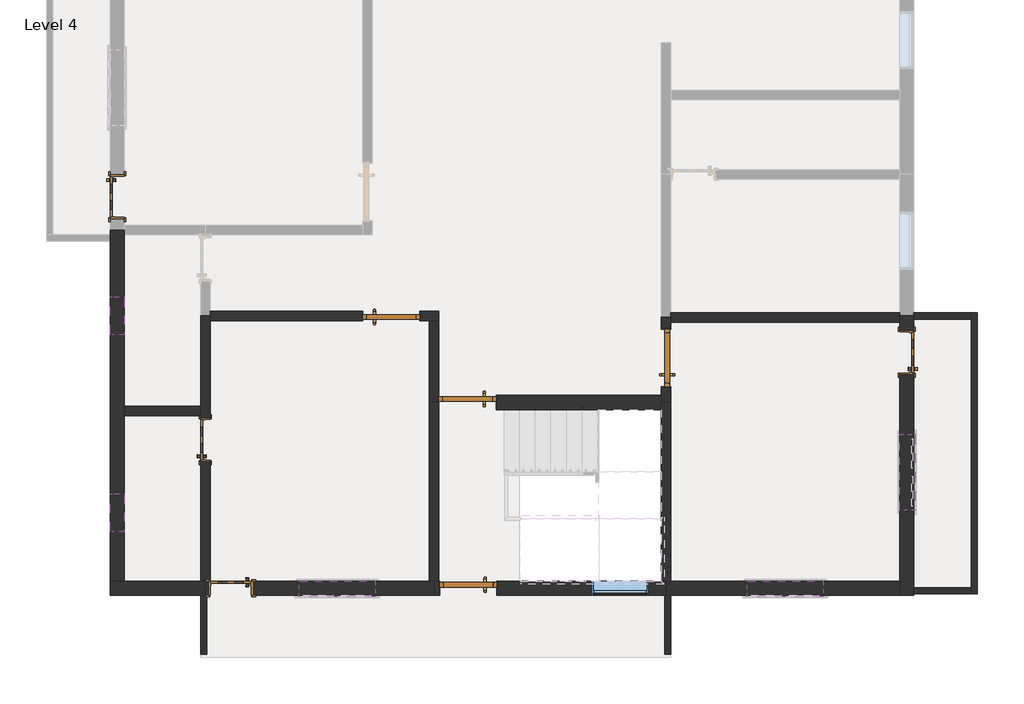
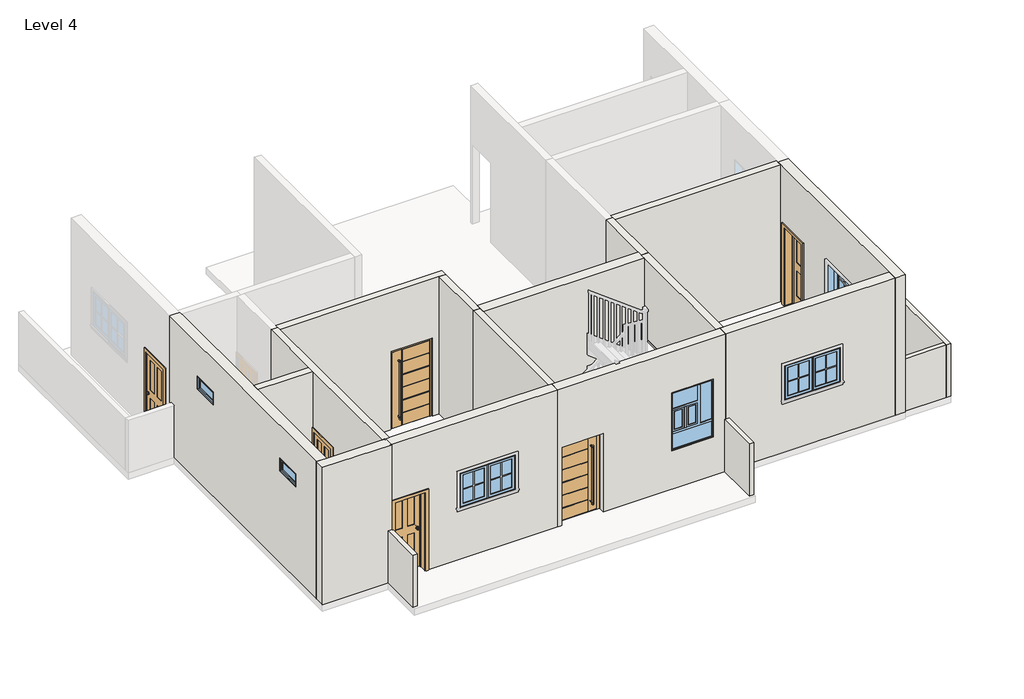
# One storey, part 1 of 3: 20 walls, 8 doors, 6 windows.
"""IFC4 building model written with IfcOpenShell, lengths in millimetres."""

from ifc_helpers import new_model, si_unit, frame, origin, place, context, project, spatial, polyline, outline, extrude, faceted_brep, transform, mapped, element, save
from components import door_3_44036f4b, door_3_3562bf2b, door_a03dd1d4, door_a34dad57, m_fixed_2_dd9f9b20, m_window_awning_double_horizontal_4_8afcb0b2, m_window_casement_double_sash_variable_3_661e274a

model = new_model("IFC4")

# Units and contexts
model_context = context("Model", 3, world=origin())
ifc_project = project(units=[si_unit("LENGTHUNIT", "METRE", prefix="MILLI")], contexts=[model_context])

# Site, building, storey
site = spatial("IfcSite", under=ifc_project)
building = spatial("IfcBuilding", under=site)
storey = spatial("IfcBuildingStorey", under=building, Name="Level 4", Elevation=9601.2)

# Doors
placement = place(None, origin())
door_3_shape = door_3_44036f4b(model_context)
element("IfcDoor", 1, ObjectType="3'", at=placement, inside=storey, context=model_context, shape_type="MappedRepresentation", body=[
    mapped(door_3_shape, transform((-13795.5794909, -9.3618509, 9601.2), x_axis=(1.0, 0.0, 0.0), y_axis=(0.0, 1.0, 0.0), z_axis=(0.0, 0.0, 1.0))),
])
element("IfcDoor", 2, ObjectType="3'", at=placement, inside=storey, context=model_context, shape_type="MappedRepresentation", body=[
    mapped(door_3_shape, transform((-9401.3794909, -682.4618509, 9601.2), x_axis=(0.0, 1.0, 0.0), y_axis=(-1.0, 0.0, 0.0), z_axis=(0.0, 0.0, 1.0))),
])
door_3_2_shape = door_3_3562bf2b(model_context)
element("IfcDoor", 3, ObjectType="3'", at=placement, inside=storey, context=model_context, shape_type="MappedRepresentation", body=[
    mapped(door_3_2_shape, transform((-12576.3794909, -1393.6618509, 9601.2), x_axis=(-1.0, 0.0, 0.0), y_axis=(0.0, -1.0, 0.0), z_axis=(0.0, 0.0, 1.0))),
])
element("IfcDoor", 4, ObjectType="3'", at=placement, inside=storey, context=model_context, shape_type="MappedRepresentation", body=[
    mapped(door_3_2_shape, transform((-12563.6794909, -4365.4618509, 9601.2), x_axis=(-1.0, 0.0, 0.0), y_axis=(0.0, -1.0, 0.0), z_axis=(0.0, 0.0, 1.0))),
])
door_shape = door_a03dd1d4(model_context)
element("IfcDoor", 5, ObjectType="M_Door-Interior-Single-4_Panel-Wood : 2'2\"", at=placement, inside=storey, context=model_context, shape_type="MappedRepresentation", body=[
    mapped(door_shape, transform((-16770.5544909, -1990.1618509, 9601.2), x_axis=(0.0, 1.0, 0.0), y_axis=(-1.0, 0.0, 0.0), z_axis=(0.0, 0.0, 1.0))),
])
door_2_shape = door_a34dad57(model_context)
element("IfcDoor", 6, ObjectType="M_Door-Interior-Single-4_Panel-Wood : 2'2\"", at=placement, inside=storey, context=model_context, shape_type="MappedRepresentation", body=[
    mapped(door_2_shape, transform((-18180.2544909, 1895.2381491, 9601.2), x_axis=(0.0, -1.0, 0.0), y_axis=(1.0, 0.0, 0.0), z_axis=(0.0, 0.0, 1.0))),
])
element("IfcDoor", 7, ObjectType="M_Door-Interior-Single-4_Panel-Wood : 2'2\"", at=placement, inside=storey, context=model_context, shape_type="MappedRepresentation", body=[
    mapped(door_2_shape, transform((-5550.1044909, -593.1618509, 9601.2), x_axis=(0.0, 1.0, 0.0), y_axis=(-1.0, 0.0, 0.0), z_axis=(0.0, 0.0, 1.0))),
])
element("IfcDoor", 8, ObjectType="M_Door-Interior-Single-4_Panel-Wood : 2'2\"", at=placement, inside=storey, context=model_context, shape_type="MappedRepresentation", body=[
    mapped(door_2_shape, transform((-16361.3794909, -4362.2868509, 9601.2), x_axis=(-1.0, 0.0, 0.0), y_axis=(0.0, -1.0, 0.0), z_axis=(0.0, 0.0, 1.0))),
])

# Walls
element("IfcWall", 9, ObjectType="Generic - 4\"", at=placement, inside=storey, context=model_context, shape_type="Brep", body=[
    faceted_brep([(-9325.1794909, -5419.5618509, 9601.2), (-9325.1794909, -4479.7618509, 9601.2), (-9325.1794909, -4479.7618509, 10820.4), (-9325.1794909, -5419.5618509, 10820.4), (-9426.7794909, -5419.5618509, 9601.2), (-9426.7794909, -5419.5618509, 10820.4), (-9426.7794909, -4479.7618509, 10820.4), (-9426.7794909, -4479.7618509, 9601.2), (-9401.3794909, -4479.7618509, 9601.2)], [[[0, 1, 2, 3]], [[4, 5, 6, 7]], [[1, 0, 4, 7, 8]], [[3, 2, 6, 5]], [[0, 3, 5, 4]], [[2, 1, 8, 7, 6]]]),
])
element("IfcWall", 10, ObjectType="Generic - 4\"", at=placement, inside=storey, context=model_context, shape_type="Brep", body=[
    faceted_brep([(-4422.9794909, -4454.3618509, 9601.2), (-4422.9794909, 41.4381491, 9601.2), (-4422.9794909, 41.4381491, 10820.4), (-4422.9794909, -4454.3618509, 10820.4), (-4524.5794909, -4454.3618509, 9601.2), (-4524.5794909, -4454.3618509, 10820.4), (-4524.5794909, -4352.7618509, 10820.4), (-4524.5794909, -60.1618509, 10820.4), (-4524.5794909, 41.4381491, 10820.4), (-4524.5794909, 41.4381491, 9601.2), (-4524.5794909, -60.1618509, 9601.2), (-4524.5794909, -4352.7618509, 9601.2)], [[[0, 1, 2, 3]], [[4, 5, 6, 7, 8, 9, 10, 11]], [[1, 0, 4, 11, 10, 9]], [[3, 2, 8, 7, 6, 5]], [[0, 3, 5, 4]], [[2, 1, 9, 8]]]),
])
element("IfcWall", 11, ObjectType="Generic - 4\"", at=placement, inside=storey, context=model_context, shape_type="SweptSolid", body=[
    extrude(outline(polyline([(-4524.5794909, -4454.3618509), (-5438.9794909, -4454.3618509), (-5438.9794909, -4352.7618509), (-4524.5794909, -4352.7618509), (-4524.5794909, -4454.3618509)])), frame((0.0, 0.0, 9601.2), z_axis=(0.0, 0.0, 1.0), x_axis=(1.0, 0.0, 0.0)), (0.0, 0.0, 1.0), 1219.2),
])
element("IfcWall", 12, ObjectType="Generic - 4\"", at=placement, inside=storey, context=model_context, shape_type="Brep", body=[
    faceted_brep([(-16843.5794909, -4479.7618509, 9601.2), (-16843.5794909, -5419.5618509, 9601.2), (-16843.5794909, -5419.5618509, 10820.4), (-16843.5794909, -4479.7618509, 10820.4), (-16741.9794909, -4479.7618509, 9601.2), (-16741.9794909, -4479.7618509, 10820.4), (-16741.9794909, -5419.5618509, 10820.4), (-16741.9794909, -5419.5618509, 9601.2), (-16792.7794909, -4479.7618509, 9601.2), (-16767.3794909, -4479.7618509, 9601.2)], [[[0, 1, 2, 3]], [[4, 5, 6, 7]], [[1, 0, 8, 9, 4, 7]], [[2, 1, 7, 6]], [[3, 2, 6, 5]], [[0, 3, 5, 4, 9, 8]]]),
])
element("IfcWall", 13, ObjectType="Generic - 4\"", at=placement, inside=storey, context=model_context, shape_type="Brep", body=[
    faceted_brep([(-4524.5794909, 41.4381491, 9601.2), (-5438.9794909, 41.4381491, 9601.2), (-5438.9794909, 41.4381491, 10820.4), (-4524.5794909, 41.4381491, 10820.4), (-4524.5794909, -60.1618509, 9601.2), (-4524.5794909, -60.1618509, 10820.4), (-5438.9794909, -60.1618509, 10820.4), (-5438.9794909, -60.1618509, 9601.2), (-5438.9794909, -34.7618509, 9601.2), (-5438.9794909, -9.3618509, 9601.2)], [[[0, 1, 2, 3]], [[4, 5, 6, 7]], [[1, 0, 4, 7, 8, 9]], [[3, 2, 6, 5]], [[0, 3, 5, 4]], [[2, 1, 9, 8, 7, 6]]]),
])
element("IfcWall", 14, ObjectType="Generic - 6\"", at=placement, inside=storey, context=model_context, shape_type="Brep", body=[
    faceted_brep([(-16691.1794909, -9.3618509, 9601.2), (-16691.1794909, -9.3618509, 12801.6), (-16691.1794909, -85.5618509, 12801.6), (-16691.1794909, -4251.1618509, 12801.6), (-16691.1794909, -4251.1618509, 9601.2), (-16691.1794909, -2345.3618509, 9601.2), (-16691.1794909, -2345.3618509, 11455.0), (-16691.1794909, -1634.9618509, 11455.0), (-16691.1794909, -1634.9618509, 9601.2), (-16691.1794909, -85.5618509, 9601.2), (-16843.5794909, -9.3618509, 12801.6), (-16843.5794909, -9.3618509, 9601.2), (-16843.5794909, -1457.1618509, 9601.2), (-16843.5794909, -1609.5618509, 9601.2), (-16843.5794909, -1634.9618509, 9601.2), (-16843.5794909, -1634.9618509, 11455.0), (-16843.5794909, -2345.3618509, 11455.0), (-16843.5794909, -2345.3618509, 9601.2), (-16843.5794909, -4251.1618509, 9601.2), (-16843.5794909, -4251.1618509, 12801.6), (-16843.5794909, -1609.5618509, 12801.6), (-16843.5794909, -1457.1618509, 12801.6), (-16716.5794909, -4251.1618509, 9601.2), (-16767.3794909, -4251.1618509, 9601.2), (-16792.7794909, -4251.1618509, 9601.2), (-16792.7794909, -4251.1618509, 12801.6), (-16767.3794909, -4251.1618509, 12801.6)], [[[0, 1, 2, 3, 4, 5, 6, 7, 8, 9]], [[10, 11, 12, 13, 14, 15, 16, 17, 18, 19, 20, 21]], [[4, 22, 23, 24, 18, 17, 5]], [[11, 0, 9, 8, 14, 13, 12]], [[1, 0, 11, 10]], [[3, 2, 1, 10, 21, 20, 19, 25, 26]], [[7, 15, 14, 8]], [[15, 7, 6, 16]], [[16, 6, 5, 17]], [[3, 26, 25, 19, 18, 24, 23, 22, 4]]]),
])
element("IfcWall", 15, ObjectType="Generic - 6\"", at=placement, inside=storey, context=model_context, shape_type="SweptSolid", body=[
    extrude(outline(polyline([(-16843.5794909, -1609.5618509), (-18062.7794909, -1609.5618509), (-18062.7794909, -1457.1618509), (-16843.5794909, -1457.1618509), (-16843.5794909, -1609.5618509)])), frame((0.0, 0.0, 9601.2), z_axis=(0.0, 0.0, 1.0), x_axis=(1.0, 0.0, 0.0)), (0.0, 0.0, 1.0), 3200.4),
])
element("IfcWall", 16, ObjectType="Generic - 6\"", at=placement, inside=storey, context=model_context, shape_type="Brep", body=[
    faceted_brep([(-13033.5794909, -85.5618509, 12801.6), (-13185.9794909, -85.5618509, 12801.6), (-16691.1794909, -85.5618509, 12801.6), (-16691.1794909, -85.5618509, 9601.2), (-14252.7794909, -85.5618509, 9601.2), (-14252.7794909, -85.5618509, 11430.0), (-13338.3794909, -85.5618509, 11430.0), (-13338.3794909, -85.5618509, 9601.2), (-13185.9794909, -85.5618509, 9601.2), (-13033.5794909, -85.5618509, 9601.2), (-16691.1794909, 66.8381491, 12801.6), (-13033.5794909, 66.8381491, 12801.6), (-13033.5794909, 66.8381491, 9601.2), (-13338.3794909, 66.8381491, 9601.2), (-13338.3794909, 66.8381491, 11430.0), (-14252.7794909, 66.8381491, 11430.0), (-14252.7794909, 66.8381491, 9601.2), (-16691.1794909, 66.8381491, 9601.2), (-13338.3794909, -65.5618509, 9601.2), (-13323.3794909, -65.5618509, 9601.2), (-13323.3794909, 11.4381491, 9601.2), (-13338.3794909, 11.4381491, 9601.2), (-16691.1794909, -9.3618509, 9601.2), (-14252.7794909, 11.4381491, 9601.2), (-14267.7794909, 11.4381491, 9601.2), (-14267.7794909, -65.5618509, 9601.2), (-14252.7794909, -65.5618509, 9601.2), (-16691.1794909, -9.3618509, 12801.6), (-14252.7794909, -65.5618509, 11430.0), (-13338.3794909, -65.5618509, 11430.0), (-13338.3794909, 11.4381491, 11430.0), (-14252.7794909, 11.4381491, 11430.0), (-14267.7794909, -65.5618509, 11445.0), (-14267.7794909, 11.4381491, 11445.0), (-13323.3794909, 11.4381491, 11445.0), (-13323.3794909, -65.5618509, 11445.0)], [[[0, 1, 2, 3, 4, 5, 6, 7, 8, 9]], [[10, 11, 12, 13, 14, 15, 16, 17]], [[12, 9, 8, 7, 18, 19, 20, 21, 13]], [[3, 22, 17, 16, 23, 24, 25, 26, 4]], [[2, 1, 0, 11, 10, 27]], [[3, 2, 27, 10, 17, 22]], [[0, 9, 12, 11]], [[5, 28, 29, 6]], [[14, 30, 31, 15]], [[6, 29, 18, 7]], [[30, 14, 13, 21]], [[28, 5, 4, 26]], [[15, 31, 23, 16]], [[32, 33, 34, 35]], [[35, 34, 20, 19]], [[31, 30, 21, 20, 34, 33, 24, 23]], [[33, 32, 25, 24]], [[29, 28, 26, 25, 32, 35, 19, 18]]]),
])
element("IfcWall", 17, ObjectType="Generic - 6\"", at=placement, inside=storey, context=model_context, shape_type="Brep", body=[
    faceted_brep([(-13185.9794909, -85.5618509, 9601.2), (-13185.9794909, -1393.6618509, 9601.2), (-13185.9794909, -1393.6618509, 12801.6), (-13185.9794909, -85.5618509, 12801.6), (-13033.5794909, -85.5618509, 12801.6), (-13033.5794909, -1279.3618509, 12801.6), (-13033.5794909, -1393.6618509, 12801.6), (-13033.5794909, -1393.6618509, 11430.0), (-13033.5794909, -1393.6618509, 9601.2), (-13033.5794909, -1376.3618508, 9601.2), (-13033.5794909, -1376.3618508, 11430.0), (-13033.5794909, -1376.3618508, 11445.0), (-13033.5794909, -1299.3618508, 11445.0), (-13033.5794909, -1299.3618508, 11430.0), (-13033.5794909, -1299.3618508, 9601.2), (-13033.5794909, -1279.3618508, 9601.2), (-13033.5794909, -85.5618509, 9601.2), (-13048.5794909, -1299.3618508, 9601.2), (-13048.5794909, -1376.3618508, 9601.2), (-13048.5794909, -1376.3618508, 11445.0), (-13048.5794909, -1299.3618508, 11445.0)], [[[0, 1, 2, 3]], [[4, 5, 6, 7, 8, 9, 10, 11, 12, 13, 14, 15, 16]], [[1, 0, 16, 15, 14, 17, 18, 9, 8]], [[2, 1, 8, 7, 6]], [[3, 2, 6, 5, 4]], [[0, 3, 4, 16]], [[19, 20, 12, 11]], [[20, 19, 18, 17]], [[18, 19, 11, 10, 9]], [[20, 17, 14, 13, 12]]]),
])
element("IfcWall", 18, ObjectType="Generic - 6\"", at=placement, inside=storey, context=model_context, shape_type="Brep", body=[
    faceted_brep([(-9325.1794909, -4251.1618509, 12801.6), (-9325.1794909, -4251.1618509, 9601.2), (-9325.1794909, -1393.6618509, 9601.2), (-9325.1794909, -1393.6618509, 12801.6), (-9477.5794909, -4251.1618509, 9601.2), (-9477.5794909, -4251.1618509, 12801.6), (-9477.5794909, -1507.9618509, 12801.6), (-9477.5794909, -1393.6618509, 12801.6), (-9477.5794909, -1393.6618509, 9601.2), (-9477.5794909, -1507.9618509, 9601.2), (-9401.3794909, -4251.1618509, 9601.2), (-9401.3794909, -4251.1618509, 12801.6)], [[[0, 1, 2, 3]], [[4, 5, 6, 7, 8, 9]], [[2, 1, 10, 4, 9, 8]], [[3, 2, 8, 7]], [[0, 3, 7, 6, 5, 11]], [[0, 11, 5, 4, 10, 1]]]),
])
element("IfcWall", 19, ObjectType="Generic - 6\"", at=placement, inside=storey, context=model_context, shape_type="Brep", body=[
    faceted_brep([(-5667.5794909, 41.4381491, 12801.6), (-5667.5794909, 41.4381491, 9601.2), (-9325.1794909, 41.4381491, 9601.2), (-9325.1794909, 41.4381491, 12801.6), (-5667.5794909, -110.9618509, 9601.2), (-5667.5794909, -110.9618509, 12801.6), (-9325.1794909, -110.9618509, 12801.6), (-9325.1794909, -110.9618509, 9601.2), (-5667.5794909, -9.3618509, 9601.2), (-5667.5794909, -34.7618509, 9601.2), (-9325.1794909, -34.7618509, 9601.2), (-9325.1794909, -34.7618509, 12801.6), (-5667.5794909, -34.7618509, 12801.6), (-5667.5794909, -9.3618509, 12801.6)], [[[0, 1, 2, 3]], [[4, 5, 6, 7]], [[2, 1, 8, 9, 4, 7, 10]], [[0, 3, 11, 6, 5, 12, 13]], [[3, 2, 10, 7, 6, 11]], [[0, 13, 12, 5, 4, 9, 8, 1]]]),
])
element("IfcWall", 20, ObjectType="Generic - 6\"", at=placement, inside=storey, context=model_context, shape_type="Brep", body=[
    faceted_brep([(-9325.1794909, -34.7618509, 9601.2), (-9325.1794909, -34.7618509, 12801.6), (-9325.1794909, -110.9618509, 12801.6), (-9325.1794909, -1393.6618509, 12801.6), (-9325.1794909, -1393.6618509, 9601.2), (-9325.1794909, -1139.6618509, 9601.2), (-9325.1794909, -1139.6618509, 11430.0), (-9325.1794909, -225.2618509, 11430.0), (-9325.1794909, -225.2618509, 9601.2), (-9325.1794909, -110.9618509, 9601.2), (-9477.5794909, -34.7618509, 12801.6), (-9477.5794909, -34.7618509, 9601.2), (-9477.5794909, -225.2618509, 9601.2), (-9477.5794909, -225.2618509, 11430.0), (-9477.5794909, -1139.6618509, 11430.0), (-9477.5794909, -1139.6618509, 9601.2), (-9477.5794909, -1279.3618509, 9601.2), (-9477.5794909, -1393.6618509, 9601.2), (-9477.5794909, -1393.6618509, 12801.6), (-9477.5794909, -1279.3618509, 12801.6), (-9345.1794909, -225.2618509, 9601.2), (-9345.1794909, -210.2618509, 9601.2), (-9422.1794909, -210.2618509, 9601.2), (-9422.1794909, -225.2618509, 9601.2), (-9422.1794909, -1139.6618509, 9601.2), (-9422.1794909, -1154.6618509, 9601.2), (-9345.1794909, -1154.6618509, 9601.2), (-9345.1794909, -1139.6618509, 9601.2), (-9345.1794909, -1139.6618509, 11430.0), (-9345.1794909, -225.2618509, 11430.0), (-9422.1794909, -225.2618509, 11430.0), (-9422.1794909, -1139.6618509, 11430.0), (-9345.1794909, -1154.6618509, 11445.0), (-9422.1794909, -1154.6618509, 11445.0), (-9422.1794909, -210.2618509, 11445.0), (-9345.1794909, -210.2618509, 11445.0)], [[[0, 1, 2, 3, 4, 5, 6, 7, 8, 9]], [[10, 11, 12, 13, 14, 15, 16, 17, 18, 19]], [[11, 0, 9, 8, 20, 21, 22, 23, 12]], [[4, 17, 16, 15, 24, 25, 26, 27, 5]], [[1, 0, 11, 10]], [[3, 2, 1, 10, 19, 18]], [[4, 3, 18, 17]], [[6, 28, 29, 7]], [[13, 30, 31, 14]], [[30, 13, 12, 23]], [[7, 29, 20, 8]], [[14, 31, 24, 15]], [[28, 6, 5, 27]], [[32, 33, 34, 35]], [[35, 34, 22, 21]], [[31, 30, 23, 22, 34, 33, 25, 24]], [[33, 32, 26, 25]], [[29, 28, 27, 26, 32, 35, 21, 20]]]),
])
element("IfcWall", 21, ObjectType="Generic - 6\"", at=placement, inside=storey, context=model_context, shape_type="Brep", body=[
    faceted_brep([(-13185.9794909, -1393.6618509, 9601.2), (-13185.9794909, -4251.1618509, 9601.2), (-13185.9794909, -4251.1618509, 12801.6), (-13185.9794909, -1393.6618509, 12801.6), (-13033.5794909, -1393.6618509, 12801.6), (-13033.5794909, -1507.9618509, 12801.6), (-13033.5794909, -4251.1618509, 12801.6), (-13033.5794909, -4251.1618509, 9601.2), (-13033.5794909, -1507.9618509, 9601.2), (-13033.5794909, -1393.6618509, 9601.2), (-13033.5794909, -1393.6618509, 11430.0), (-13109.7794909, -4251.1618509, 9601.2), (-13109.7794909, -4251.1618509, 12801.6)], [[[0, 1, 2, 3]], [[4, 5, 6, 7, 8, 9, 10]], [[1, 0, 9, 8, 7, 11]], [[3, 2, 12, 6, 5, 4]], [[0, 3, 4, 10, 9]], [[2, 1, 11, 7, 6, 12]]]),
])
element("IfcWall", 22, ObjectType="Generic - 9\"", at=placement, inside=storey, context=model_context, shape_type="Brep", body=[
    faceted_brep([(-5667.5794909, -4251.1618509, 12801.6), (-5667.5794909, -4251.1618509, 9601.2), (-9325.1794909, -4251.1618509, 9601.2), (-9401.3794909, -4251.1618509, 9601.2), (-9401.3794909, -4251.1618509, 12801.6), (-9325.1794909, -4251.1618509, 12801.6), (-8105.9794909, -4251.1618509, 11620.4), (-8105.9794909, -4251.1618509, 10820.4), (-6886.7794909, -4251.1618509, 10820.4), (-6886.7794909, -4251.1618509, 11620.4), (-5667.5794909, -4479.7618509, 9601.2), (-5667.5794909, -4479.7618509, 12801.6), (-9401.3794909, -4479.7618509, 12801.6), (-9401.3794909, -4479.7618509, 9601.2), (-9325.1794909, -4479.7618509, 9601.2), (-8105.9794909, -4479.7618509, 11620.4), (-6886.7794909, -4479.7618509, 11620.4), (-6886.7794909, -4479.7618509, 10820.4), (-8105.9794909, -4479.7618509, 10820.4)], [[[0, 1, 2, 3, 4, 5], [6, 7, 8, 9]], [[10, 11, 12, 13, 14], [15, 16, 17, 18]], [[3, 2, 1, 10, 14, 13]], [[4, 3, 13, 12]], [[0, 5, 4, 12, 11]], [[0, 11, 10, 1]], [[7, 6, 15, 18]], [[8, 7, 18, 17]], [[9, 8, 17, 16]], [[6, 9, 16, 15]]]),
])
element("IfcWall", 23, ObjectType="Generic - 9\"", at=placement, inside=storey, context=model_context, shape_type="Brep", body=[
    faceted_brep([(-18062.7794909, -4251.1618509, 9601.2), (-18062.7794909, -1609.5618509, 9601.2), (-18062.7794909, -1457.1618509, 9601.2), (-18062.7794909, 1286.0381491, 9601.2), (-18062.7794909, 1362.2381491, 9601.2), (-18062.7794909, 1362.2381491, 12801.6), (-18062.7794909, 1286.0381491, 12801.6), (-18062.7794909, -1457.1618509, 12801.6), (-18062.7794909, -1609.5618509, 12801.6), (-18062.7794909, -4251.1618509, 12801.6), (-18062.7794909, -3463.7618509, 11734.8), (-18062.7794909, -3463.7618509, 12039.6), (-18062.7794909, -2854.1618509, 12039.6), (-18062.7794909, -2854.1618509, 11734.8), (-18062.7794909, -314.1618509, 11734.8), (-18062.7794909, -314.1618509, 12039.6), (-18062.7794909, 295.4381491, 12039.6), (-18062.7794909, 295.4381491, 11734.8), (-18291.3794909, -4251.1618509, 9601.2), (-18291.3794909, -4251.1618509, 12801.6), (-18291.3794909, 1362.2381491, 12801.6), (-18291.3794909, 1362.2381491, 9601.2), (-18291.3794909, 1286.0381491, 9601.2), (-18291.3794909, 1184.4381491, 9601.2), (-18291.3794909, -3463.7618509, 11734.8), (-18291.3794909, -2854.1618509, 11734.8), (-18291.3794909, -2854.1618509, 12039.6), (-18291.3794909, -3463.7618509, 12039.6), (-18291.3794909, -314.1618509, 11734.8), (-18291.3794909, 295.4381491, 11734.8), (-18291.3794909, 295.4381491, 12039.6), (-18291.3794909, -314.1618509, 12039.6)], [[[0, 1, 2, 3, 4, 5, 6, 7, 8, 9], [10, 11, 12, 13], [14, 15, 16, 17]], [[18, 19, 20, 21, 22, 23], [24, 25, 26, 27], [28, 29, 30, 31]], [[4, 3, 2, 1, 0, 18, 23, 22, 21]], [[9, 8, 7, 6, 5, 20, 19]], [[0, 9, 19, 18]], [[11, 10, 24, 27]], [[12, 11, 27, 26]], [[13, 12, 26, 25]], [[10, 13, 25, 24]], [[15, 14, 28, 31]], [[16, 15, 31, 30]], [[17, 16, 30, 29]], [[14, 17, 29, 28]], [[4, 21, 20, 5]]]),
])
element("IfcWall", 24, ObjectType="Generic - 9\"", at=placement, inside=storey, context=model_context, shape_type="Brep", body=[
    faceted_brep([(-13033.5794909, -1279.3618509, 12801.6), (-9477.5794909, -1279.3618509, 12801.6), (-9477.5794909, -1279.3618509, 9601.2), (-12119.1794909, -1279.3618509, 9601.2), (-12119.1794909, -1279.3618509, 11430.0), (-13033.5794909, -1279.3618509, 11430.0), (-9477.5794909, -1507.9618509, 12801.6), (-13033.5794909, -1507.9618509, 12801.6), (-13033.5794909, -1507.9618509, 11430.0), (-12119.1794909, -1507.9618509, 11430.0), (-12119.1794909, -1507.9618509, 9601.2), (-9477.5794909, -1507.9618509, 9601.2), (-9477.5794909, -1393.6618509, 9601.2), (-12119.1794909, -1376.3618508, 9601.2), (-12104.1794909, -1376.3618508, 9601.2), (-12104.1794909, -1299.3618508, 9601.2), (-12119.1794909, -1299.3618508, 9601.2), (-13033.5794909, -1393.6618509, 12801.6), (-9477.5794909, -1393.6618509, 12801.6), (-13033.5794909, -1299.3618508, 11430.0), (-13033.5794909, -1299.3618508, 11445.0), (-13033.5794909, -1376.3618508, 11445.0), (-13033.5794909, -1376.3618508, 11430.0), (-12119.1794909, -1299.3618508, 11430.0), (-12119.1794909, -1376.3618508, 11430.0), (-12104.1794909, -1299.3618508, 11445.0), (-12104.1794909, -1376.3618508, 11445.0)], [[[0, 1, 2, 3, 4, 5]], [[6, 7, 8, 9, 10, 11]], [[2, 12, 11, 10, 13, 14, 15, 16, 3]], [[1, 0, 17, 7, 6, 18]], [[7, 17, 0, 5, 19, 20, 21, 22, 8]], [[2, 1, 18, 6, 11, 12]], [[4, 23, 19, 5]], [[22, 24, 9, 8]], [[23, 4, 3, 16]], [[9, 24, 13, 10]], [[25, 26, 21, 20]], [[24, 22, 21, 26, 14, 13]], [[26, 25, 15, 14]], [[19, 23, 16, 15, 25, 20]]]),
])
element("IfcWall", 25, ObjectType="Generic - 9\"", at=placement, inside=storey, context=model_context, shape_type="Brep", body=[
    faceted_brep([(-5667.5794909, -4479.7618509, 12801.6), (-5667.5794909, -4251.1618509, 12801.6), (-5667.5794909, -110.9618509, 12801.6), (-5667.5794909, -9.3618509, 12801.6), (-5667.5794909, -9.3618509, 9601.2), (-5667.5794909, -110.9618509, 9601.2), (-5667.5794909, -237.9618509, 9601.2), (-5667.5794909, -237.9618509, 11455.0), (-5667.5794909, -948.3618509, 11455.0), (-5667.5794909, -948.3618509, 9601.2), (-5667.5794909, -4251.1618509, 9601.2), (-5667.5794909, -4479.7618509, 9601.2), (-5667.5794909, -3120.0618509, 11620.4), (-5667.5794909, -3120.0618509, 10820.4), (-5667.5794909, -1900.8618509, 10820.4), (-5667.5794909, -1900.8618509, 11620.4), (-5438.9794909, -9.3618509, 12801.6), (-5438.9794909, -4479.7618509, 12801.6), (-5438.9794909, -4479.7618509, 9601.2), (-5438.9794909, -4454.3618509, 9601.2), (-5438.9794909, -4352.7618509, 9601.2), (-5438.9794909, -948.3618509, 9601.2), (-5438.9794909, -948.3618509, 11455.0), (-5438.9794909, -237.9618509, 11455.0), (-5438.9794909, -237.9618509, 9601.2), (-5438.9794909, -60.1618509, 9601.2), (-5438.9794909, -9.3618509, 9601.2), (-5438.9794909, -3120.0618509, 11620.4), (-5438.9794909, -1900.8618509, 11620.4), (-5438.9794909, -1900.8618509, 10820.4), (-5438.9794909, -3120.0618509, 10820.4)], [[[0, 1, 2, 3, 4, 5, 6, 7, 8, 9, 10, 11], [12, 13, 14, 15]], [[16, 17, 18, 19, 20, 21, 22, 23, 24, 25, 26], [27, 28, 29, 30]], [[4, 26, 25, 24, 6, 5]], [[18, 11, 10, 9, 21, 20, 19]], [[3, 2, 1, 0, 17, 16]], [[11, 18, 17, 0]], [[12, 15, 28, 27]], [[15, 14, 29, 28]], [[14, 13, 30, 29]], [[13, 12, 27, 30]], [[3, 16, 26, 4]], [[23, 7, 6, 24]], [[7, 23, 22, 8]], [[8, 22, 21, 9]]]),
])
element("IfcWall", 26, ObjectType="Generic - 9\"", at=placement, inside=storey, context=model_context, shape_type="Brep", body=[
    faceted_brep([(-13109.7794909, -4251.1618509, 9601.2), (-13109.7794909, -4251.1618509, 12801.6), (-13033.5794909, -4251.1618509, 12801.6), (-9477.5794909, -4251.1618509, 12801.6), (-9401.3794909, -4251.1618509, 12801.6), (-9401.3794909, -4251.1618509, 9601.2), (-9477.5794909, -4251.1618509, 9601.2), (-12106.4794909, -4251.1618509, 9601.2), (-12106.4794909, -4251.1618509, 11430.0), (-13020.8794909, -4251.1618509, 11430.0), (-13020.8794909, -4251.1618509, 9601.2), (-13033.5794909, -4251.1618509, 9601.2), (-10595.1794909, -4251.1618509, 11851.2), (-10595.1794909, -4251.1618509, 10501.2), (-9680.7794909, -4251.1618509, 10501.2), (-9680.7794909, -4251.1618509, 11851.2), (-13109.7794909, -4479.7618509, 12801.6), (-13109.7794909, -4479.7618509, 9601.2), (-13020.8794909, -4479.7618509, 9601.2), (-13020.8794909, -4479.7618509, 11430.0), (-12106.4794909, -4479.7618509, 11430.0), (-12106.4794909, -4479.7618509, 9601.2), (-9426.7794909, -4479.7618509, 9601.2), (-9401.3794909, -4479.7618509, 9601.2), (-9401.3794909, -4479.7618509, 12801.6), (-10595.1794909, -4479.7618509, 11851.2), (-9680.7794909, -4479.7618509, 11851.2), (-9680.7794909, -4479.7618509, 10501.2), (-10595.1794909, -4479.7618509, 10501.2), (-12106.4794909, -4348.1618508, 9601.2), (-12091.4794909, -4348.1618508, 9601.2), (-12091.4794909, -4271.1618508, 9601.2), (-12106.4794909, -4271.1618508, 9601.2), (-13020.8794909, -4271.1618508, 9601.2), (-13035.8794909, -4271.1618508, 9601.2), (-13035.8794909, -4348.1618508, 9601.2), (-13020.8794909, -4348.1618508, 9601.2), (-12106.4794909, -4271.1618508, 11430.0), (-13020.8794909, -4271.1618508, 11430.0), (-13020.8794909, -4348.1618508, 11430.0), (-12106.4794909, -4348.1618508, 11430.0), (-12091.4794909, -4271.1618508, 11445.0), (-12091.4794909, -4348.1618508, 11445.0), (-13035.8794909, -4348.1618508, 11445.0), (-13035.8794909, -4271.1618508, 11445.0)], [[[0, 1, 2, 3, 4, 5, 6, 7, 8, 9, 10, 11], [12, 13, 14, 15]], [[16, 17, 18, 19, 20, 21, 22, 23, 24], [25, 26, 27, 28]], [[5, 23, 22, 21, 29, 30, 31, 32, 7, 6]], [[17, 0, 11, 10, 33, 34, 35, 36, 18]], [[1, 0, 17, 16]], [[4, 3, 2, 1, 16, 24]], [[8, 37, 38, 9]], [[19, 39, 40, 20]], [[39, 19, 18, 36]], [[9, 38, 33, 10]], [[20, 40, 29, 21]], [[37, 8, 7, 32]], [[41, 42, 43, 44]], [[44, 43, 35, 34]], [[40, 39, 36, 35, 43, 42, 30, 29]], [[42, 41, 31, 30]], [[38, 37, 32, 31, 41, 44, 34, 33]], [[12, 15, 26, 25]], [[15, 14, 27, 26]], [[14, 13, 28, 27]], [[13, 12, 25, 28]], [[4, 24, 23, 5]]]),
])
element("IfcWall", 27, ObjectType="Generic - 9\"", at=placement, inside=storey, context=model_context, shape_type="Brep", body=[
    faceted_brep([(-16792.7794909, -4251.1618509, 12801.6), (-16691.1794909, -4251.1618509, 12801.6), (-13185.9794909, -4251.1618509, 12801.6), (-13109.7794909, -4251.1618509, 12801.6), (-13109.7794909, -4251.1618509, 9601.2), (-13185.9794909, -4251.1618509, 9601.2), (-16006.1794909, -4251.1618509, 9601.2), (-16006.1794909, -4251.1618509, 11455.0), (-16716.5794909, -4251.1618509, 11455.0), (-16716.5794909, -4251.1618509, 9601.2), (-16792.7794909, -4251.1618509, 9601.2), (-15269.5794909, -4251.1618509, 11620.4), (-15269.5794909, -4251.1618509, 10820.4), (-14050.3794909, -4251.1618509, 10820.4), (-14050.3794909, -4251.1618509, 11620.4), (-13109.7794909, -4479.7618509, 12801.6), (-16792.7794909, -4479.7618509, 12801.6), (-16792.7794909, -4479.7618509, 9601.2), (-16741.9794909, -4479.7618509, 9601.2), (-16716.5794909, -4479.7618509, 9601.2), (-16716.5794909, -4479.7618509, 11455.0), (-16006.1794909, -4479.7618509, 11455.0), (-16006.1794909, -4479.7618509, 9601.2), (-13109.7794909, -4479.7618509, 9601.2), (-15269.5794909, -4479.7618509, 11620.4), (-14050.3794909, -4479.7618509, 11620.4), (-14050.3794909, -4479.7618509, 10820.4), (-15269.5794909, -4479.7618509, 10820.4)], [[[0, 1, 2, 3, 4, 5, 6, 7, 8, 9, 10], [11, 12, 13, 14]], [[15, 16, 17, 18, 19, 20, 21, 22, 23], [24, 25, 26, 27]], [[17, 10, 9, 19, 18]], [[4, 23, 22, 6, 5]], [[3, 2, 1, 0, 16, 15]], [[4, 3, 15, 23]], [[11, 14, 25, 24]], [[14, 13, 26, 25]], [[13, 12, 27, 26]], [[12, 11, 24, 27]], [[8, 20, 19, 9]], [[20, 8, 7, 21]], [[21, 7, 6, 22]], [[10, 17, 16, 0]]]),
])
element("IfcWall", 28, ObjectType="Generic - 9\"", at=placement, inside=storey, context=model_context, shape_type="Brep", body=[
    faceted_brep([(-16767.3794909, -4251.1618509, 12801.6), (-16767.3794909, -4251.1618509, 9601.2), (-16843.5794909, -4251.1618509, 9601.2), (-18062.7794909, -4251.1618509, 9601.2), (-18291.3794909, -4251.1618509, 9601.2), (-18291.3794909, -4251.1618509, 12801.6), (-18062.7794909, -4251.1618509, 12801.6), (-16843.5794909, -4251.1618509, 12801.6), (-16767.3794909, -4479.7618509, 9601.2), (-16767.3794909, -4479.7618509, 12801.6), (-18291.3794909, -4479.7618509, 12801.6), (-18291.3794909, -4479.7618509, 9601.2), (-16843.5794909, -4479.7618509, 9601.2)], [[[0, 1, 2, 3, 4, 5, 6, 7]], [[8, 9, 10, 11, 12]], [[4, 3, 2, 1, 8, 12, 11]], [[0, 7, 6, 5, 10, 9]], [[5, 4, 11, 10]], [[0, 9, 8, 1]]]),
])

# Windows
m_fixed_2_shape = m_fixed_2_dd9f9b20(model_context)
element("IfcWindow", 29, ObjectType="M_Fixed : 2'", at=placement, inside=storey, context=model_context, shape_type="MappedRepresentation", body=[
    mapped(m_fixed_2_shape, transform((-18164.0794909, -3158.9618509, 10819.8), x_axis=(0.0, 1.0, 0.0), y_axis=(-1.0, 0.0, 0.0), z_axis=(0.0, 0.0, 1.0))),
])
element("IfcWindow", 30, ObjectType="M_Fixed : 2'", at=placement, inside=storey, context=model_context, shape_type="MappedRepresentation", body=[
    mapped(m_fixed_2_shape, transform((-18164.0794909, -9.3618509, 10819.8), x_axis=(0.0, 1.0, 0.0), y_axis=(-1.0, 0.0, 0.0), z_axis=(0.0, 0.0, 1.0))),
])
m_window_awning_double_horizontal_4_shape = m_window_awning_double_horizontal_4_8afcb0b2(model_context)
element("IfcWindow", 31, ObjectType="M_Window-Awning-Double-Horizontal : 4'", at=placement, inside=storey, context=model_context, shape_type="MappedRepresentation", body=[
    mapped(m_window_awning_double_horizontal_4_shape, transform((-14659.9794909, -4365.4618509, 9920.4), x_axis=(-1.0, 0.0, 0.0), y_axis=(0.0, -1.0, 0.0), z_axis=(0.0, 0.0, 1.0))),
])
element("IfcWindow", 32, ObjectType="M_Window-Awning-Double-Horizontal : 4'", at=placement, inside=storey, context=model_context, shape_type="MappedRepresentation", body=[
    mapped(m_window_awning_double_horizontal_4_shape, transform((-5553.2794909, -2510.4618509, 9920.4), x_axis=(0.0, -1.0, 0.0), y_axis=(1.0, 0.0, 0.0), z_axis=(0.0, 0.0, 1.0))),
])
element("IfcWindow", 33, ObjectType="M_Window-Awning-Double-Horizontal : 4'", at=placement, inside=storey, context=model_context, shape_type="MappedRepresentation", body=[
    mapped(m_window_awning_double_horizontal_4_shape, transform((-7496.3794909, -4365.4618509, 9920.4), x_axis=(-1.0, 0.0, 0.0), y_axis=(0.0, -1.0, 0.0), z_axis=(0.0, 0.0, 1.0))),
])
m_window_casement_double_sash_variable_3_shape = m_window_casement_double_sash_variable_3_661e274a(model_context)
element("IfcWindow", 34, ObjectType="M_Window-Casement-Double-Sash-Variable : 3'", at=placement, inside=storey, context=model_context, shape_type="MappedRepresentation", body=[
    mapped(m_window_casement_double_sash_variable_3_shape, transform((-10137.9794909, -4365.4618509, 9601.2), x_axis=(-1.0, 0.0, 0.0), y_axis=(0.0, -1.0, 0.0), z_axis=(0.0, 0.0, 1.0))),
])

save(model, "model.ifc")

# Revit data of these elements
# Type "3'"
#   Type Mark = "41"
#   Water resistance = "up to Class E900, EN 12208:2001"
#   Uniclass2015Version = "v1.21"
#   Uniclass2015Reference = "Ss_25_30_20_30"
#   Uniclass2015Description = "Frame and door leaf system"
#   URL = "www.aluprof.com"
#   Type IFC Predefined Type = "USERDEFINED"
#   Right-hand / Left-hand door [instance default] = ""
#   Resistance to wind load = "up to Class C5/B5, EN 12210:2001"
#   Insert type = "ST"
#   Hardware [instance default] = ""
#   Product page = "https://aluprof.com/en/architects/offer/window-and-door-systems/panel-doors#visualisation"
#   Operation = "SinglePanelOutwardOpening"
#   Opening type = "Outward"
#   NBSReference = "25-50-20/125"
#   NBSDescription = "Frame and door leaf system"
#   Important = "The actual acceptable construction dimensions are dependent on the selection of profiles and hardware, glazing type, construction weight and the construction’s operating conditions. These should be determined by a suitably qualified person, and using ALUPROF’s calculation software"
#   IfcExportType = "USERDEFINED"
#   IfcExportAs = "IfcDoorType"
#   Handle type [instance default] = ""
#   Manufacturer = "ALUPROF SA"
#   Export Type to IFC As = "IfcDoorType"
#   Door sill type [instance default] = ""
#   Description = "External single-leaf panel door outward opening"
#   Model = "MB-86 ST Panel Door AD07"
#   Content of the recyclate in the material = "69.2%"
#   COBie.Type.WarrantyDurationParts = ""
#   COBie.Type.Name = ""
#   COBie.Type.Manufacturer = "ALUPROF SA"
#   COBie.Space.Name = ""
#   COBie.Floor.Name = ""
#   COBie.Facility.Name = ""
#   COBie.CreatedOn = ""
#   COBie.Component.WarrantyStartDate = ""
#   COBie.Component.Name = "MB-86 ST Panel Door AD07"
#   Burglar resistance = "RC2"
#   Air permeability = "up to Class 4, EN 12207:2001"
#   Width of the active leaf = 2' - 8.17717"
#   Placement in wall = 0' - 0.7874"
#   Thickness = 0' - 3.0315"
#   Height of the opening sash = 5' - 9.44094"
#   Handle Offset = 3' - 5.33858"
#   Rough Height = 6' - 2.40945"
#   Rough Width = 3' - 1.1811"
#   Height = 6' - 0"
#   Width = 3' - 0"
#   Construction depth = 0' - 3.0315"
#   Clear opening width = 2' - 3.94882"
#   Clear opening height = 5' - 8.47638"
#   Height of the array = 0' - 11.08136"
#   Schedule No. [instance default] = 1
#   Handrail [instance default] = yes
#   IsExternal = yes
#   Handle [instance default] = no
#   Door closer [instance default] = no
#   Function = 1
#   COBie.Type = yes
#   COBie = yes
#   Access control [instance default] = no
#   Panel = element 361060
#   Wall Closure = (empty or 0)
# Type "M_Door-Interior-Single-4_Panel-Wood : 2'2\""
#   Type Mark = "43"
#   Assembly Code = "C1020300"
#   Analytic Construction = "Wooden"
#   Top Rail = 0' - 4.72441"
#   Thickness = 0' - 1.37795"
#   Thermal Resistance (R) = 0.455703 (m²·K)/W
#   Swing Angle [instance default] = 90.00°
#   Stiles = 0' - 4.72441"
#   Rough Width = 2' - 3.9685"
#   Rough Height = 6' - 0.98425"
#   Mullion = 0' - 4.52756"
#   Lock Rail = 0' - 7.87402"
#   Height = 6' - 0"
#   Width = 2' - 2"
#   Heat Transfer Coefficient (U) = 2.19465 W/(m²·K)
#   Bottom Rail = 0' - 9.05512"
#   Trim Material = Cherry
#   Panel Material = Cherry
#   Frame Material = Cherry
#   Door Handle Material = Aluminum
#   Visual Light Transmittance = 0
#   Solar Heat Gain Coefficient = 0
#   Wall Closure = (empty or 0)
#   Function = (empty or 0)
# Type "Generic - 4\""
#   Layers, outside or top first: 0' - 4" no material (function 1)
# Type "Generic - 6\""
#   Layers, outside or top first: 0' - 6" no material (function 1)
# Type "Generic - 9\""
#   Layers, outside or top first: 0' - 9" no material (function 1)
# Type "M_Fixed : 2'"
#   Type Mark = "37"
#   Construction Type Id = "GSP4R"
#   Analytic Construction = "1/8 in Pilkington single glazing"
#   Visual Light Transmittance = 0.9
#   Thermal Resistance (R) = 0.271106 (m²·K)/W
#   Solar Heat Gain Coefficient = 0.78
#   Heat Transfer Coefficient (U) = 3.6886 W/(m²·K)
#   Height = 1' - 0"
#   Default Sill Height = 3' - 0.02362"
#   Width = 2' - 0"
#   Window Inset = 0' - 0.74803"
#   Define Thermal Properties by = 1
#   Frame Exterior Material = Sash
#   Frame Interior Material = Sash
#   Glass Pane Material = Glass
#   Sash = Sash
#   Wall Closure = (empty or 0)
# Type "M_Window-Awning-Double-Horizontal : 4'"
#   Type Mark = "28"
#   Fire Rating = "0.5h"
#   Assembly Code = "B2020100"
#   Analytic Construction = "Double glazing - domestic"
#   Window Inset [instance default] = 0' - 0"
#   Wall Thickness [instance default] = 0' - 5.90551"
#   Interior Wall Closure [instance default] = 0' - 2.15551"
#   Half Width = 2' - 0"
#   Visual Light Transmittance = 0.81
#   Thermal Resistance (R) = 0.319569 (m²·K)/W
#   Solar Heat Gain Coefficient = 0.76
#   Rough Width = 4' - 0.59055"
#   Rough Height = 2' - 8.08661"
#   Height = 2' - 7.49606"
#   Heat Transfer Coefficient (U) = 3.12929 W/(m²·K)
#   Frame Extension [instance default] = 0' - 0 1/4"
#   Exterior Wall Closure [instance default] = 0' - 1 1/4"
#   Extension Jamb [instance default] = 0' - 2.15551"
#   Default Sill Height = 2' - 11.43307"
#   Width = 4' - 0"
#   Muntin Visibility = yes
#   Interior Trim Visibility [instance default] = yes
#   Exterior Trim Visibility [instance default] = yes
#   Extension Jamb Visibility [instance default] = yes
#   Interior Trim Material = Wood - Stained
#   Muntin Pattern = M_Muntin Pattern_2x2 : M_Muntin Pattern_2x2
#   Interior Trim = M_Trim-Window-Interior-Flat : Picture Frame
#   Interior Frame Material = Wood - Stained
#   Glass Panel Material = Glass
#   Exterior Trim Material = Clad - White
#   Exterior Trim = M_Trim-Window-Exterior-Flat : with Sill
#   Exterior Frame Material = Clad - White
#   Wall Closure = (empty or 0)
# Type "M_Window-Casement-Double-Sash-Variable : 3'"
#   Type Mark = "36"
#   Fire Rating = "0.5h"
#   Assembly Code = "B2020100"
#   Analytic Construction = "Double glazing - domestic"
#   Window Inset [instance default] = 0' - 0 5/8"
#   Wall Thickness [instance default] = 0' - 5.90551"
#   Visual Light Transmittance = 0.81
#   Transom Height Ratio = 0.3
#   Transom Height = 1' - 3.94488"
#   Thermal Resistance (R) = 0.319569 (m²·K)/W
#   Solar Heat Gain Coefficient = 0.76
#   Rough Width = 3' - 0.59055"
#   Rough Height = 4' - 5.74016"
#   Opening Window Height = 1' - 9.25984"
#   Heat Transfer Coefficient (U) = 3.12929 W/(m²·K)
#   Height = 4' - 5.14961"
#   Frame Gap 3 [instance default] = 0' - 1.65041"
#   Frame Gap 2 [instance default] = 0' - 0.62598"
#   Frame Gap 1 = 0' - 1 51/128"
#   Window Width = 1' - 0"
#   Default Sill Height = 2' - 11.43307"
#   Width = 3' - 0"
#   Frame Material = Metal - Aluminum
#   Glass Panel Material = Glass
#   Wall Closure = (empty or 0)
# Elements 1, 2, 3, 4 (IfcDoor, "3'")
#   Right-hand / Left-hand door = ""
#   Hardware = ""
#   Handle type = ""
#   Door sill type = ""
#   Schedule No. = 1
#   Handrail = yes
#   Handle = no
#   Door closer = no
#   Access control = no
#   Phase Created = New Construction
# Elements 5, 6, 7, 8 (IfcDoor, "M_Door-Interior-Single-4_Panel-Wood : 2'2\"")
#   Swing Angle = 90.00°
#   Phase Created = New Construction
#   Materials on its faces: "Cherry", "Aluminum"
# Elements 9, 11, 12, 13 (IfcWall, "Generic - 4\"")
#   Top Offset = 0' - 0"
#   Base Offset = 0' - 0"
#   Unconnected Height = 4' - 0"
#   wall height = 4' - 0"
#   Phase Created = New Construction
#   Base Constraint = Level 4
#   Materials on its faces: "Default Wall", "WALL2"
# Element 10 (IfcWall, "Generic - 4\"")
#   Top Offset = 0' - 0"
#   Base Offset = 0' - 0"
#   Unconnected Height = 4' - 0"
#   wall height = 4' - 0"
#   Phase Created = New Construction
#   Base Constraint = Level 4
#   Materials on its faces: "WALL2", "Default Wall"
# Element 14 (IfcWall, "Generic - 6\"")
#   Top Offset = 0' - 0"
#   Base Offset = 0' - 0"
#   Unconnected Height = 10' - 6"
#   wall height = 10' - 6"
#   Phase Created = New Construction
#   Base Constraint = Level 4
#   Materials on its faces: "Default Wall", "BED ROOM WALL 2", "BATH ROOM WALL 1"
# Element 15 (IfcWall, "Generic - 6\"")
#   Top Offset = 0' - 0"
#   Base Offset = 0' - 0"
#   Unconnected Height = 10' - 6"
#   wall height = 10' - 6"
#   Phase Created = New Construction
#   Base Constraint = Level 4
#   Materials on its faces: "Default Wall", "BATH ROOM WALL 1"
# Element 16 (IfcWall, "Generic - 6\"")
#   Top Offset = 0' - 0"
#   Base Offset = 0' - 0"
#   Unconnected Height = 10' - 6"
#   wall height = 10' - 6"
#   Phase Created = New Construction
#   Base Constraint = Level 4
#   Materials on its faces: "Default Wall", "LIVING 2", "BED ROOM WALL1"
# Elements 17, 20 (IfcWall, "Generic - 6\"")
#   Top Offset = 0' - 0"
#   Base Offset = 0' - 0"
#   Unconnected Height = 10' - 6"
#   wall height = 10' - 6"
#   Phase Created = New Construction
#   Base Constraint = Level 4
#   Materials on its faces: "Default Wall", "BED ROOM WALL 2", "LIVING 2"
# Elements 18, 21 (IfcWall, "Generic - 6\"")
#   Top Offset = 0' - 0"
#   Base Offset = 0' - 0"
#   Unconnected Height = 10' - 6"
#   wall height = 10' - 6"
#   Phase Created = New Construction
#   Base Constraint = Level 4
#   Materials on its faces: "Default Wall", "BED ROOM WALL 2", "LIVING"
# Element 19 (IfcWall, "Generic - 6\"")
#   Top Offset = 0' - 0"
#   Base Offset = 0' - 0"
#   Unconnected Height = 10' - 6"
#   wall height = 10' - 6"
#   Phase Created = New Construction
#   Base Constraint = Level 4
#   Materials on its faces: "Default Wall", "LIVING", "BED ROOM WALL1"
# Element 22 (IfcWall, "Generic - 9\"")
#   Top Offset = 0' - 0"
#   Base Offset = 0' - 0"
#   Unconnected Height = 10' - 6"
#   wall height = 10' - 6"
#   Phase Created = New Construction
#   Base Constraint = Level 4
#   Materials on its faces: "Default Wall", "BED ROOM WALL 2", "WALL2"
# Element 23 (IfcWall, "Generic - 9\"")
#   Top Offset = 0' - 0"
#   Base Offset = 0' - 0"
#   Unconnected Height = 10' - 6"
#   wall height = 10' - 6"
#   Phase Created = New Construction
#   Base Constraint = Level 4
#   Materials on its faces: "Default Wall", "BATH ROOM WALL 1", "WALL2"
# Element 24 (IfcWall, "Generic - 9\"")
#   Top Offset = 0' - 0"
#   Base Offset = 0' - 0"
#   Unconnected Height = 10' - 6"
#   wall height = 10' - 6"
#   Phase Created = New Construction
#   Base Constraint = Level 4
#   Materials on its faces: "Default Wall", "LIVING 2", "LIVING"
# Element 25 (IfcWall, "Generic - 9\"")
#   Top Offset = 0' - 0"
#   Base Offset = 0' - 0"
#   Unconnected Height = 10' - 6"
#   wall height = 10' - 6"
#   Phase Created = New Construction
#   Base Constraint = Level 4
#   Materials on its faces: "Default Wall", "WALL2", "BED ROOM WALL1"
# Element 26 (IfcWall, "Generic - 9\"")
#   Top Offset = 0' - 0"
#   Base Offset = 0' - 0"
#   Unconnected Height = 10' - 6"
#   wall height = 10' - 6"
#   Phase Created = New Construction
#   Base Constraint = Level 4
#   Materials on its faces: "Default Wall", "LIVING", "WALL2"
# Element 27 (IfcWall, "Generic - 9\"")
#   Top Offset = 0' - 0"
#   Base Offset = 0' - 0"
#   Unconnected Height = 10' - 6"
#   wall height = 10' - 6"
#   Phase Created = New Construction
#   Base Constraint = Level 4
#   Materials on its faces: "Default Wall", "BED ROOM WALL1", "WALL2"
# Element 28 (IfcWall, "Generic - 9\"")
#   Top Offset = 0' - 0"
#   Base Offset = 0' - 0"
#   Unconnected Height = 10' - 6"
#   wall height = 10' - 6"
#   Phase Created = New Construction
#   Base Constraint = Level 4
#   Materials on its faces: "Default Wall", "WALL2"
# Element 29 (IfcWindow, "M_Fixed : 2'")
#   Mark = "43"
#   Phase Created = New Construction
#   Materials on its faces: "Sash", "Glass"
# Element 30 (IfcWindow, "M_Fixed : 2'")
#   Mark = "44"
#   Phase Created = New Construction
#   Materials on its faces: "Sash", "Glass"
# Element 31 (IfcWindow, "M_Window-Awning-Double-Horizontal : 4'")
#   Mark = "34"
#   Window Inset = 0' - 0"
#   Interior Wall Closure = 0' - 2.15551"
#   Frame Extension = 0' - 0 1/4"
#   Exterior Wall Closure = 0' - 1 1/4"
#   Interior Trim Visibility = yes
#   Exterior Trim Visibility = yes
#   Phase Created = New Construction
#   Materials on its faces: "Wood - Stained", "Glass", "Clad - White"
# Element 32 (IfcWindow, "M_Window-Awning-Double-Horizontal : 4'")
#   Mark = "38"
#   Window Inset = 0' - 0"
#   Interior Wall Closure = 0' - 2.15551"
#   Frame Extension = 0' - 0 1/4"
#   Exterior Wall Closure = 0' - 1 1/4"
#   Interior Trim Visibility = yes
#   Exterior Trim Visibility = yes
#   Phase Created = New Construction
#   Materials on its faces: "Wood - Stained", "Glass", "Clad - White"
# Element 33 (IfcWindow, "M_Window-Awning-Double-Horizontal : 4'")
#   Mark = "39"
#   Window Inset = 0' - 0"
#   Interior Wall Closure = 0' - 2.15551"
#   Frame Extension = 0' - 0 1/4"
#   Exterior Wall Closure = 0' - 1 1/4"
#   Interior Trim Visibility = yes
#   Exterior Trim Visibility = yes
#   Phase Created = New Construction
#   Materials on its faces: "Wood - Stained", "Glass", "Clad - White"
# Element 34 (IfcWindow, "M_Window-Casement-Double-Sash-Variable : 3'")
#   Mark = "40"
#   Window Inset = 0' - 0 5/8"
#   Frame Gap 3 = 0' - 1.65041"
#   Frame Gap 2 = 0' - 0.62598"
#   Phase Created = New Construction
#   Materials on its faces: "Metal - Aluminum", "Glass"
# Materials
#   "Cherry": class "Wood", colour RGB 226 177 128, transparency 0, Description = "Prunus Serotina", Cost = 0
#   "Aluminum": class "Metal", colour RGB 247 247 247, transparency 0, Description = "Aluminum 6061", Cost = 0
#   "Sash": class "Wood", colour RGB 224 178 126, transparency 0, Cost = 0
#   "Glass": class "Glass", colour RGB 0 128 192, transparency 0.9, Description = "Soda Lime Glass", Cost = 0
#   "Wood - Stained": class "Wood", colour RGB 224 178 126, transparency 0, Cost = 0
#   "Clad - White": class "Wood", colour RGB 242 242 238, transparency 0, Cost = 0
#   "Metal - Aluminum": class "Metal", colour RGB 247 247 247, transparency 0
#   "Default Wall": colour RGB 128 128 128, transparency 0, Cost = 0
#   "WALL2": class "Generic", colour RGB 120 120 120, transparency 0, Cost = 0
#   "BED ROOM WALL 2": class "Generic", colour RGB 120 120 120, transparency 0, Cost = 0
#   "BATH ROOM WALL 1": class "Generic", colour RGB 120 120 120, transparency 0, Cost = 0
#   "LIVING 2": class "Generic", colour RGB 120 120 120, transparency 0, Cost = 0
#   "BED ROOM WALL1": class "Generic", colour RGB 120 120 120, transparency 0, Cost = 0
#   "LIVING": class "Generic", colour RGB 120 120 120, transparency 0, Cost = 0
